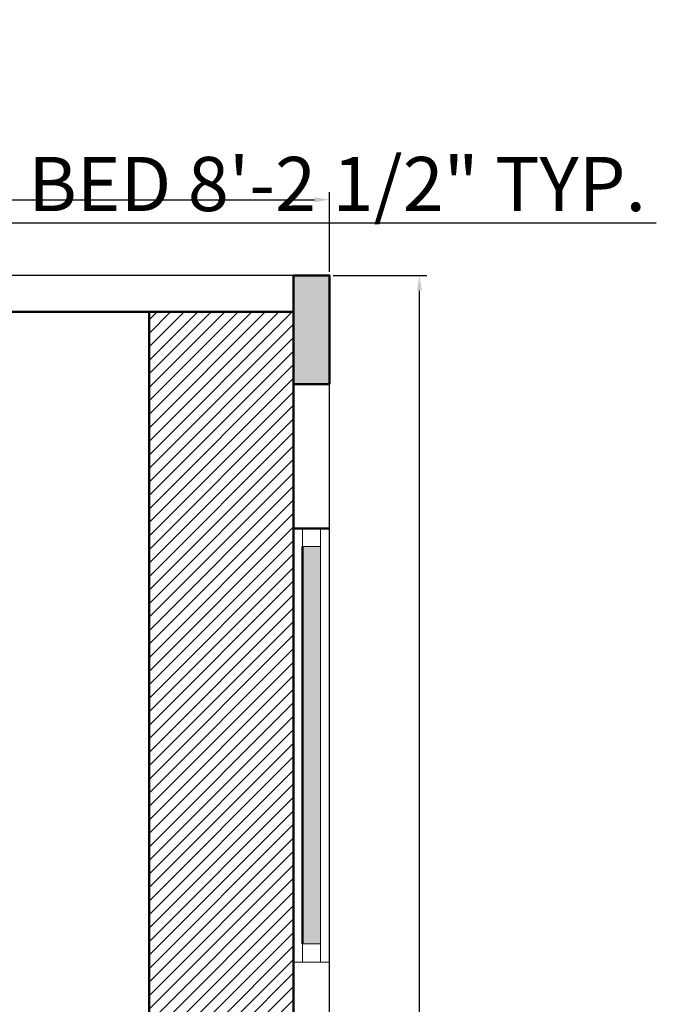
# Model space of a CAD drawing. Units: inches. Extents: x 3064 to 19385, y 846 to 15425.
# Tile 9 of 108: x 3511 to 3617, y 1275 to 1439. Entities that reach past the tile are written whole.
import ezdxf

# ---------------------------------------------------------------- set-up
doc = ezdxf.new("R2010")
doc.units = ezdxf.units.IN
for name, color, linetype, lineweight in [('A-ANNO-DIMS', 2, 'Continuous', 18), ('A-COLS', 1, 'Continuous', 35), ('A-FURN-PATT', 252, 'Continuous', 13), ('A-GLAZ', 4, 'Continuous', 18), ('A-WALL', 7, 'Continuous', 50), ('C-PROP', 6, 'Continuous', 25)]:
    doc.layers.add(name, color=color, linetype=linetype, lineweight=lineweight)
doc.styles.get("Standard").update_dxf_attribs({"font": 'arial.ttf'})
doc.dimstyles.new('ISO-25', dxfattribs={"dimtxt": 9, "dimasz": 2.5, "dimexe": 1.25, "dimexo": 0.625, "dimtad": 1, "dimdec": 1, "dimlunit": 3, "dimtxsty": 'Standard', "dimcen": 2.5, "dimadec": 0, "dimazin": 0, "dimtfac": 1, "dimtdec": 1, "dimtmove": 0, "dimatfit": 3, "dimfxl": 1, "dimarcsym": 0})

# ---------------------------------------------------------------- blocks, each defined once
blk = doc.blocks.new('*D38')
at = {"layer": 'A-ANNO-DIMS', "color": 0, "lineweight": -2, "transparency": 16777216}
for p, q in [((3220.85, 1396.96), (3220.85, 1410.2)), ((3562.85, 1396.96), (3562.85, 1410.2)), ((3223.35, 1408.95), (3560.35, 1408.95))]:
    blk.add_line(p, q, dxfattribs=at)
at = {"layer": 'A-ANNO-DIMS', "color": 0, "transparency": 16777216}
for points in [[(3223.35, 1409.36), (3223.35, 1408.53), (3220.85, 1408.95)], [(3560.35, 1409.36), (3560.35, 1408.53), (3562.85, 1408.95)]]:
    blk.add_solid(points, dxfattribs=at)
at = {"layer": 'Defpoints', "color": 0, "transparency": 16777216}
for p in [(3562.85, 1408.95), (3220.85, 1396.34), (3562.85, 1396.34)]:
    blk.add_point(p, dxfattribs=at)
at = {"layer": 'A-ANNO-DIMS', "color": 0, "transparency": 16777216, "insert": (3391.85, 1414.17), "char_height": 9, "attachment_point": 5}
blk.add_mtext('28\'-6"', dxfattribs=at)
blk = doc.blocks.new('*D42')
at = {"layer": 'A-ANNO-DIMS', "color": 0, "lineweight": -2, "transparency": 16777216}
for p, q in [((3563.47, 1396.34), (3579.02, 1396.34)), ((3577.77, 882.84), (3577.77, 1393.84)), ((3563.47, 880.34), (3579.02, 880.34))]:
    blk.add_line(p, q, dxfattribs=at)
at = {"layer": 'A-ANNO-DIMS', "color": 0, "transparency": 16777216}
for points in [[(3577.35, 1393.84), (3578.19, 1393.84), (3577.77, 1396.34)], [(3577.35, 882.84), (3578.19, 882.84), (3577.77, 880.34)]]:
    blk.add_solid(points, dxfattribs=at)
at = {"layer": 'Defpoints', "color": 0, "transparency": 16777216}
for p in [(3562.85, 1396.34), (3577.77, 1396.34), (3562.85, 880.34)]:
    blk.add_point(p, dxfattribs=at)
at = {"layer": 'A-ANNO-DIMS', "color": 0, "transparency": 16777216, "insert": (3572.55, 1138.34), "char_height": 9, "attachment_point": 5, "rotation": 90}
blk.add_mtext("43'", dxfattribs=at)
blk = doc.blocks.new('WIN-1900')
blk.add_line((3, 0), (3, 66))
blk.add_lwpolyline([(3, 66), (0, 66), (0, 69), (3, 69)], close=True)
blk = doc.blocks.new('*D401')
at = {"layer": 'A-ANNO-DIMS', "color": 0, "lineweight": -2, "transparency": 16777216}
for p, q in [((3410.1, 1390.96), (3410.1, 1406.37)), ((3508.6, 1390.96), (3508.6, 1406.37)), ((3412.6, 1405.12), (3506.1, 1405.12)), ((3508.6, 1405.12), (3617.13, 1405.12))]:
    blk.add_line(p, q, dxfattribs=at)
at = {"layer": 'A-ANNO-DIMS', "color": 0, "transparency": 16777216}
for points in [[(3412.6, 1405.53), (3412.6, 1404.7), (3410.1, 1405.12)], [(3506.1, 1405.53), (3506.1, 1404.7), (3508.6, 1405.12)]]:
    blk.add_solid(points, dxfattribs=at)
at = {"layer": 'Defpoints', "color": 0, "transparency": 16777216}
for p in [(3508.6, 1405.12), (3410.1, 1390.34), (3508.6, 1390.34)]:
    blk.add_point(p, dxfattribs=at)
at = {"layer": 'A-ANNO-DIMS', "color": 0, "transparency": 16777216, "insert": (3564.11, 1410.39), "char_height": 9, "attachment_point": 5}
blk.add_mtext('BED 8\'-2 1/2" TYP.', dxfattribs=at)

msp = doc.modelspace()

# ---------------------------------------------------------------- hatches: boundary and pattern name
at = {"layer": 'A-COLS'}
h = msp.add_hatch(color=256, dxfattribs=at)
h.dxf.hatch_style = 1
h.paths.add_polyline_path([(3556.85, 1378.34), (3562.85, 1378.34), (3562.85, 1396.34), (3556.85, 1396.34)])
at = {"layer": 'A-FURN-PATT'}
h = msp.add_hatch(dxfattribs=at)
h.set_pattern_fill('ANSI31', color=256, scale=0.5)
h.set_pattern_definition([(45, (-2094.8195, 0), (-1.122532, 1.122532), [])])
h.paths.add_polyline_path([(3532.85, 1258.34), (3556.85, 1258.34), (3556.85, 1390.34), (3532.85, 1390.34)])
at = {"layer": 'A-GLAZ'}
h = msp.add_hatch(color=256, dxfattribs=at)
h.dxf.hatch_style = 1
h.paths.add_polyline_path([(3558.35, 1285.34), (3561.35, 1285.34), (3561.35, 1351.34), (3558.35, 1351.34)])

# ---------------------------------------------------------------- linework, layer by layer
msp.add_line((3562.85, 1282.34), (3556.85, 1282.34), dxfattribs=at)
msp.add_lwpolyline([(3561.35, 1282.34), (3558.35, 1282.34), (3558.35, 1285.34), (3561.35, 1285.34)], close=True, dxfattribs=at)
at = {"layer": 'A-WALL'}
for p, q in [((3556.85, 1390.34), (3361.85, 1390.34)), ((3532.85, 1252.34), (3532.85, 1390.34)), ((3556.85, 1258.34), (3556.85, 1390.34)), ((3556.85, 1354.34), (3562.85, 1354.34)), ((3558.35, 1351.34), (3558.35, 1285.34))]:
    msp.add_line(p, q, dxfattribs=at)
msp.add_lwpolyline([(3562.85, 1378.34), (3562.85, 1396.34), (3556.85, 1396.34), (3556.85, 1378.34)], close=True, dxfattribs=at)
at = {"layer": 'C-PROP'}
for p, q in [((3562.85, 1396.34), (3220.85, 1396.34)), ((3562.85, 880.34), (3562.85, 1396.34))]:
    msp.add_line(p, q, dxfattribs=at)

# ---------------------------------------------------------------- block references
at = {"layer": 'A-GLAZ'}
msp.add_blockref('WIN-1900', (3558.35, 1285.34), dxfattribs=at)

# ---------------------------------------------------------------- dimensions: what is measured, and where the dimension line sits
at = {"layer": 'A-ANNO-DIMS'}
dim = msp.add_linear_dim(base=(3508.6, 1405.12), p1=(3410.1, 1390.34), p2=(3508.6, 1390.34), text='BED <> TYP.', dimstyle='ISO-25', override={"dimdec": 1, "dimrnd": 0, "dimzin": 1, "dimlunit": 4, "dimfrac": 2}, dxfattribs=at)
dim.commit()
dim.dimension.update_dxf_attribs({"geometry": '*D401', "text_midpoint": (3564.11, 1410.39)})
dim = msp.add_linear_dim(base=(3562.85, 1408.95), p1=(3220.85, 1396.34), p2=(3562.85, 1396.34), dimstyle='ISO-25', override={"dimclrd": 0, "dimclre": 0, "dimclrt": 0}, dxfattribs=at)
dim.commit()
dim.dimension.update_dxf_attribs({"geometry": '*D38', "text_midpoint": (3391.85, 1414.17)})
dim = msp.add_linear_dim(base=(3577.77, 1396.34), p1=(3562.85, 880.34), p2=(3562.85, 1396.34), angle=90, dimstyle='ISO-25', override={"dimclrd": 0, "dimclre": 0, "dimclrt": 0}, dxfattribs=at)
dim.commit()
dim.dimension.update_dxf_attribs({"geometry": '*D42', "text_midpoint": (3572.55, 1138.34)})

doc.saveas('drawing.dxf')
